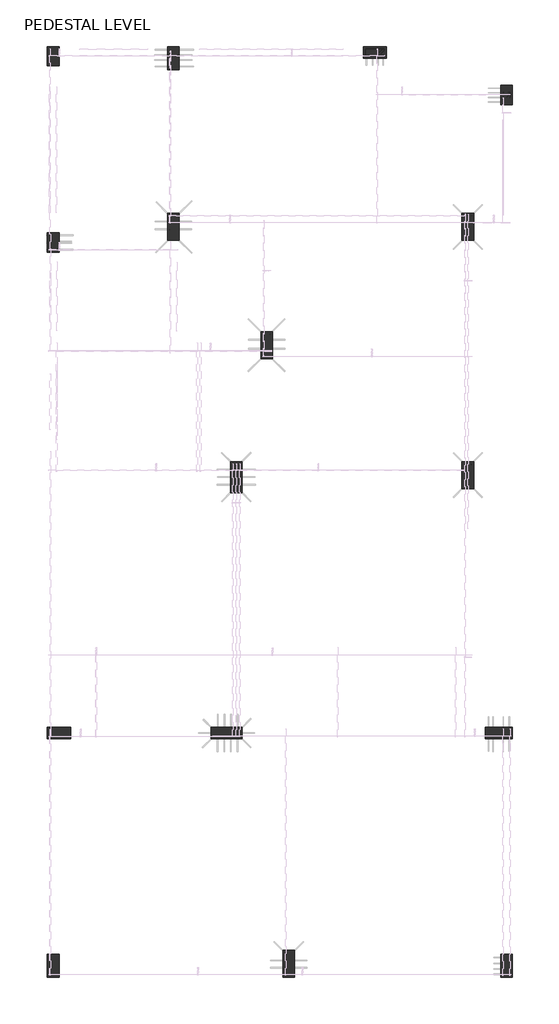
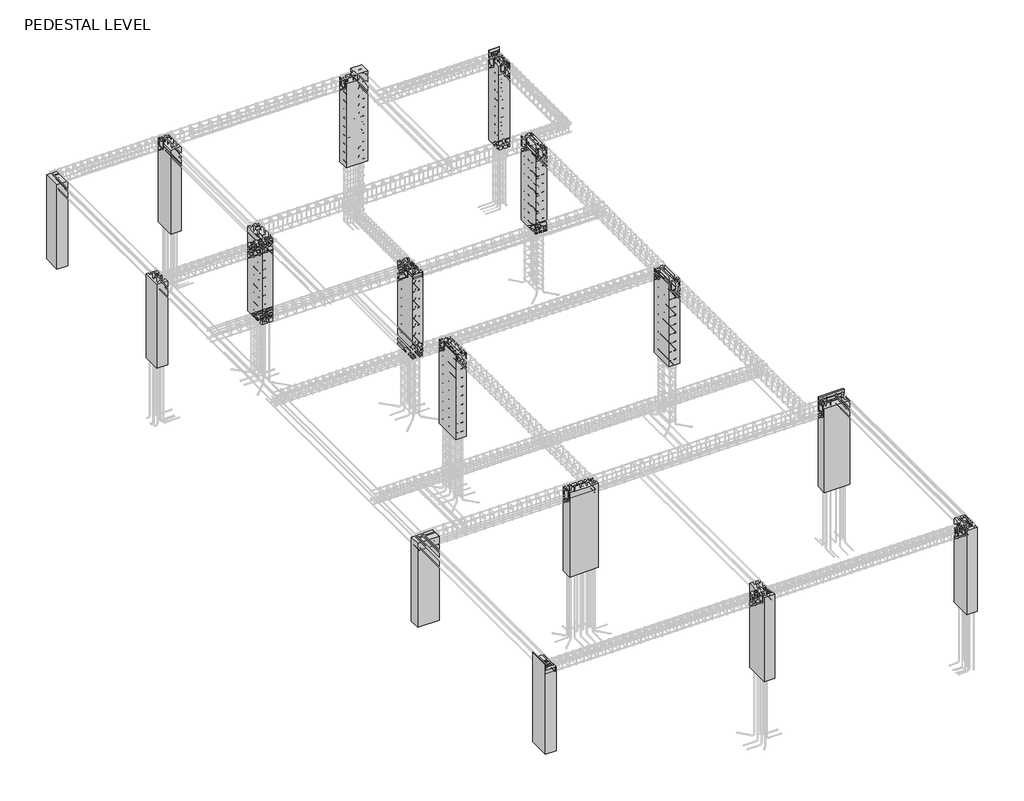
# One storey, part 1 of 8: 16 columns.
"""IFC4 building model written with IfcOpenShell, lengths in millimetres."""

from ifc_helpers import new_model, si_unit, origin, place, context, project, spatial, faceted_brep, element, save

model = new_model("IFC4")

# Units and contexts
model_context = context("Model", 3, world=origin())
ifc_project = project(units=[si_unit("LENGTHUNIT", "METRE", prefix="MILLI")], contexts=[model_context])

# Site, building, storey
site = spatial("IfcSite", under=ifc_project)
building = spatial("IfcBuilding", under=site)
storey = spatial("IfcBuildingStorey", under=building, Name="PEDESTAL LEVEL", Elevation=990.6)

# Columns
placement = place(None, origin())
element("IfcColumn", 1, ObjectType="Concrete-Rectangular-Column : C1", at=placement, inside=storey, context=model_context, shape_type="Brep", body=[
    faceted_brep([(150503.0232069, -91588.7007776, 990.6), (150503.0232069, -91969.7007776, 990.6), (150274.4232069, -91969.7007776, 990.6), (150274.4232069, -91588.7007776, 990.6), (150274.4232069, -91588.7007776, 2873.0), (150503.0232069, -91588.7007776, 2873.0), (150503.0232069, -91588.7007776, 2695.2), (150274.4232069, -91969.7007776, 2695.2), (150274.4232069, -91969.7007776, 2873.0), (150503.0232069, -91969.7007776, 2695.2), (150503.0232069, -91969.7007776, 2873.0), (150503.0232069, -91817.3007776, 2873.0)], [[[0, 1, 2, 3]], [[0, 3, 4, 5, 6]], [[3, 2, 7, 8, 4]], [[2, 1, 9, 10, 8, 7]], [[1, 0, 6, 5, 11, 10, 9]], [[5, 4, 8, 10, 11]]]),
])
element("IfcColumn", 2, ObjectType="Concrete-Rectangular-Column : C1", at=placement, inside=storey, context=model_context, shape_type="Brep", body=[
    faceted_brep([(159418.4232069, -92350.7007776, 3000.0), (159189.8232069, -92350.7007776, 3000.0), (159189.8232069, -92352.1871115, 3000.0), (159418.4232069, -92352.1871115, 3000.0), (159418.4232069, -92350.7007776, 990.6), (159418.4232069, -92731.7007776, 990.6), (159189.8232069, -92731.7007776, 990.6), (159189.8232069, -92350.7007776, 990.6), (159189.8232069, -92350.7007776, 2695.2), (159189.8232069, -92731.7007776, 2873.0), (159189.8232069, -92579.3007776, 2873.0), (159189.8232069, -92352.1871115, 2873.0), (159418.4232069, -92731.7007776, 2873.0), (159418.4232069, -92352.1871115, 2873.0)], [[[0, 1, 2, 3]], [[4, 5, 6, 7]], [[1, 0, 4, 7, 8]], [[7, 6, 9, 10, 11, 2, 1, 8]], [[6, 5, 12, 9]], [[5, 4, 0, 3, 13, 12]], [[13, 11, 10, 9, 12]], [[11, 13, 3, 2]]]),
])
element("IfcColumn", 3, ObjectType="Concrete-Rectangular-Column : C1", at=placement, inside=storey, context=model_context, shape_type="Brep", body=[
    faceted_brep([(150503.0232069, -95246.3007776, 990.6), (150503.0232069, -95627.3007776, 990.6), (150274.4232069, -95627.3007776, 990.6), (150274.4232069, -95246.3007776, 990.6), (150274.4232069, -95246.3007776, 2695.2), (150274.4232069, -95246.3007776, 2873.0), (150503.0232069, -95246.3007776, 2873.0), (150503.0232069, -95246.3007776, 2695.2), (150274.4232069, -95627.3007776, 2695.2), (150274.4232069, -95627.3007776, 2873.0), (150274.4232069, -95398.7007776, 2873.0), (150503.0232069, -95627.3007776, 2695.2), (150503.0232069, -95627.3007776, 2873.0), (150503.0232069, -95398.7007776, 2873.0)], [[[0, 1, 2, 3]], [[0, 3, 4, 5, 6, 7]], [[3, 2, 8, 9, 10, 5, 4]], [[2, 1, 11, 12, 9, 8]], [[1, 0, 7, 6, 13, 12, 11]], [[9, 12, 13, 6, 5, 10]]]),
])
element("IfcColumn", 4, ObjectType="Concrete-Rectangular-Column : C2", at=placement, inside=storey, context=model_context, shape_type="Brep", body=[
    faceted_brep([(152865.2232069, -91588.7007776, 990.6), (152865.2232069, -92045.9007776, 990.6), (152636.6232069, -92045.9007776, 990.6), (152636.6232069, -91588.7007776, 990.6), (152636.6232069, -91588.7007776, 2695.2), (152636.6232069, -91588.7007776, 2873.0), (152865.2232069, -91588.7007776, 2873.0), (152865.2232069, -91588.7007776, 2695.2), (152636.6232069, -92045.9007776, 2619.0), (152636.6232069, -92045.9007776, 2873.0), (152636.6232069, -91817.3007776, 2873.0), (152865.2232069, -92045.9007776, 2619.0), (152865.2232069, -92045.9007776, 2873.0), (152865.2232069, -91817.3007776, 2873.0)], [[[0, 1, 2, 3]], [[0, 3, 4, 5, 6, 7]], [[3, 2, 8, 9, 10, 5, 4]], [[2, 1, 11, 12, 9, 8]], [[1, 0, 7, 6, 13, 12, 11]], [[6, 5, 10, 9, 12, 13]]]),
])
element("IfcColumn", 5, ObjectType="Concrete-Rectangular-Column : C2", at=placement, inside=storey, context=model_context, shape_type="Brep", body=[
    faceted_brep([(156941.4384274, -91817.3007776, 3000.0), (156941.4384274, -91588.7007776, 3000.0), (156713.3232069, -91588.7007776, 3000.0), (156713.3232069, -91817.3007776, 3000.0), (156484.2384274, -91588.7007776, 990.6), (156941.4384274, -91588.7007776, 990.6), (156941.4384274, -91817.3007776, 990.6), (156484.2384274, -91817.3007776, 990.6), (156484.2384274, -91817.3007776, 2695.2), (156484.2384274, -91817.3007776, 2873.0), (156484.2384274, -91588.7007776, 2873.0), (156484.2384274, -91588.7007776, 2695.2), (156941.4384274, -91817.3007776, 2695.2), (156713.3232069, -91817.3007776, 2873.0), (156941.4384274, -91588.7007776, 2695.2), (156713.3232069, -91588.7007776, 2873.0)], [[[0, 1, 2, 3]], [[4, 5, 6, 7]], [[4, 7, 8, 9, 10, 11]], [[7, 6, 12, 0, 3, 13, 9, 8]], [[1, 0, 12, 6, 5, 14]], [[5, 4, 11, 10, 15, 2, 1, 14]], [[13, 15, 10, 9]], [[15, 13, 3, 2]]]),
])
element("IfcColumn", 6, ObjectType="Concrete-Rectangular-Column : C2", at=placement, inside=storey, context=model_context, shape_type="Brep", body=[
    faceted_brep([(150274.4232069, -104961.8007776, 990.6), (150731.6232069, -104961.8007776, 990.6), (150731.6232069, -105190.4007776, 990.6), (150274.4232069, -105190.4007776, 990.6), (150274.4232069, -105190.4007776, 2695.2), (150274.4232069, -105190.4007776, 2873.0), (150274.4232069, -104961.8007776, 2873.0), (150274.4232069, -104961.8007776, 2619.0), (150731.6232069, -105190.4007776, 2619.0), (150731.6232069, -105190.4007776, 2873.0), (150503.0232069, -105190.4007776, 2873.0), (150277.1537731, -105190.4007776, 2873.0), (150731.6232069, -104961.8007776, 2619.0), (150731.6232069, -104961.8007776, 2873.0), (150503.0232069, -104961.8007776, 2873.0)], [[[0, 1, 2, 3]], [[0, 3, 4, 5, 6, 7]], [[3, 2, 8, 9, 10, 11, 5, 4]], [[2, 1, 12, 13, 9, 8]], [[1, 0, 7, 6, 14, 13, 12]], [[6, 5, 11, 10, 9, 13, 14]]]),
])
element("IfcColumn", 7, ObjectType="Concrete-Rectangular-Column : C2", at=placement, inside=storey, context=model_context, shape_type="Brep", body=[
    faceted_brep([(159418.4232069, -109419.5007776, 990.6), (159418.4232069, -109876.7007776, 990.6), (159189.8232069, -109876.7007776, 990.6), (159189.8232069, -109419.5007776, 990.6), (159189.8232069, -109419.5007776, 2695.2), (159189.8232069, -109419.5007776, 2873.0), (159418.4232069, -109419.5007776, 2873.0), (159418.4232069, -109419.5007776, 2695.2), (159189.8232069, -109876.7007776, 2695.2), (159189.8232069, -109876.7007776, 2873.0), (159189.8232069, -109648.1007776, 2873.0), (159418.4232069, -109876.7007776, 2873.0)], [[[0, 1, 2, 3]], [[0, 3, 4, 5, 6, 7]], [[3, 2, 8, 9, 10, 5, 4]], [[2, 1, 11, 9, 8]], [[1, 0, 7, 6, 11]], [[6, 5, 10, 9, 11]]]),
])
element("IfcColumn", 8, ObjectType="Concrete-Rectangular-Column : C2", at=placement, inside=storey, context=model_context, shape_type="Brep", body=[
    faceted_brep([(150274.4232069, -109419.5007776, 3000.0), (150274.4232069, -109876.7007776, 3000.0), (150277.1537731, -109876.7007776, 3000.0), (150277.1537731, -109419.5007776, 3000.0), (150503.0232069, -109419.5007776, 990.6), (150503.0232069, -109876.7007776, 990.6), (150274.4232069, -109876.7007776, 990.6), (150274.4232069, -109419.5007776, 990.6), (150274.4232069, -109419.5007776, 2695.2), (150277.1537731, -109419.5007776, 2873.0), (150503.0232069, -109419.5007776, 2873.0), (150503.0232069, -109419.5007776, 2695.2), (150503.0232069, -109876.7007776, 2695.2), (150503.0232069, -109876.7007776, 2873.0), (150277.1537731, -109876.7007776, 2873.0), (150503.0232069, -109648.1007776, 2873.0)], [[[0, 1, 2, 3]], [[4, 5, 6, 7]], [[4, 7, 8, 0, 3, 9, 10, 11]], [[1, 0, 8, 7, 6]], [[6, 5, 12, 13, 14, 2, 1]], [[5, 4, 11, 10, 15, 13, 12]], [[9, 14, 13, 15, 10]], [[14, 9, 3, 2]]]),
])
element("IfcColumn", 9, ObjectType="Concrete-Rectangular-Column : C3", at=placement, inside=storey, context=model_context, shape_type="Brep", body=[
    faceted_brep([(158656.423207, -94865.3007776, 990.6), (158656.423207, -95398.7007776, 990.6), (158427.823207, -95398.7007776, 990.6), (158427.823207, -94865.3007776, 990.6), (158427.823207, -94865.3007776, 2619.0), (158427.823207, -94865.3007776, 2873.0), (158656.423207, -94865.3007776, 2873.0), (158656.423207, -94865.3007776, 2695.2), (158427.823207, -95398.7007776, 2619.0), (158427.823207, -95398.7007776, 2873.0), (158427.823207, -95093.9007776, 2873.0), (158656.423207, -95398.7007776, 2619.0), (158656.423207, -95398.7007776, 2873.0), (158656.423207, -95093.9007776, 2873.0)], [[[0, 1, 2, 3]], [[0, 3, 4, 5, 6, 7]], [[3, 2, 8, 9, 10, 5, 4]], [[2, 1, 11, 12, 9, 8]], [[1, 0, 7, 6, 13, 12, 11]], [[6, 5, 10, 9, 12, 13]]]),
])
element("IfcColumn", 10, ObjectType="Concrete-Rectangular-Column : C3", at=placement, inside=storey, context=model_context, shape_type="Brep", body=[
    faceted_brep([(158656.423207, -99742.1007776, 990.6), (158656.423207, -100275.5007776, 990.6), (158427.823207, -100275.5007776, 990.6), (158427.823207, -99742.1007776, 990.6), (158427.823207, -99742.1007776, 2619.0), (158427.823207, -99742.1007776, 2695.2), (158427.823207, -99742.1007776, 2873.0), (158656.423207, -99742.1007776, 2873.0), (158656.423207, -99742.1007776, 2619.0), (158427.823207, -100275.5007776, 2619.0), (158427.823207, -100275.5007776, 2873.0), (158427.823207, -99970.7007776, 2873.0), (158656.423207, -100275.5007776, 2619.0), (158656.423207, -100275.5007776, 2873.0), (158656.423207, -99970.7007776, 2873.0)], [[[0, 1, 2, 3]], [[0, 3, 4, 5, 6, 7, 8]], [[3, 2, 9, 10, 11, 6, 5, 4]], [[2, 1, 12, 13, 10, 9]], [[1, 0, 8, 7, 14, 13, 12]], [[7, 6, 11, 10, 13, 14]]]),
])
element("IfcColumn", 11, ObjectType="Concrete-Rectangular-Column : C3", at=placement, inside=storey, context=model_context, shape_type="Brep", body=[
    faceted_brep([(159418.4232069, -104961.8007776, 3000.0), (158885.0232069, -104961.8007776, 3000.0), (158885.0232069, -105001.8007776, 3000.0), (159418.4232069, -105001.8007776, 3000.0), (158885.0232069, -104961.8007776, 990.6), (159418.4232069, -104961.8007776, 990.6), (159418.4232069, -105190.4007776, 990.6), (158885.0232069, -105190.4007776, 990.6), (158885.0232069, -105190.4007776, 2619.0), (158885.0232069, -105190.4007776, 2873.0), (158885.0232069, -105001.8007776, 2873.0), (158885.0232069, -104961.8007776, 2619.0), (159418.4232069, -105190.4007776, 2873.0), (159418.4232069, -105001.8007776, 2873.0)], [[[0, 1, 2, 3]], [[4, 5, 6, 7]], [[4, 7, 8, 9, 10, 2, 1, 11]], [[7, 6, 12, 9, 8]], [[6, 5, 0, 3, 13, 12]], [[1, 0, 5, 4, 11]], [[13, 10, 9, 12]], [[10, 13, 3, 2]]]),
])
element("IfcColumn", 12, ObjectType="Concrete-Rectangular-Column : C4", at=placement, inside=storey, context=model_context, shape_type="Brep", body=[
    faceted_brep([(152865.2232069, -94865.3007776, 990.6), (152865.2232069, -95398.7007776, 990.6), (152636.6232069, -95398.7007776, 990.6), (152636.6232069, -94865.3007776, 990.6), (152636.6232069, -94865.3007776, 2619.0), (152636.6232069, -94865.3007776, 2873.0), (152865.2232069, -94865.3007776, 2873.0), (152865.2232069, -94865.3007776, 2619.0), (152636.6232069, -95398.7007776, 2695.2), (152636.6232069, -95398.7007776, 2873.0), (152636.6232069, -95093.9007776, 2873.0), (152865.2232069, -95398.7007776, 2695.2), (152865.2232069, -95398.7007776, 2873.0), (152865.2232069, -95093.9007776, 2873.0)], [[[0, 1, 2, 3]], [[0, 3, 4, 5, 6, 7]], [[3, 2, 8, 9, 10, 5, 4]], [[2, 1, 11, 12, 9, 8]], [[1, 0, 7, 6, 13, 12, 11]], [[6, 5, 10, 9, 12, 13]]]),
])
element("IfcColumn", 13, ObjectType="Concrete-Rectangular-Column : C4", at=placement, inside=storey, context=model_context, shape_type="Brep", body=[
    faceted_brep([(154699.7805846, -97189.4007776, 990.6), (154699.7805846, -97722.8007776, 990.6), (154471.1805846, -97722.8007776, 990.6), (154471.1805846, -97189.4007776, 990.6), (154471.1805846, -97189.4007776, 2695.2), (154471.1805846, -97189.4007776, 2873.0), (154699.7805846, -97189.4007776, 2873.0), (154699.7805846, -97189.4007776, 2695.2), (154471.1805846, -97722.8007776, 2873.0), (154699.7805846, -97722.8007776, 2695.2), (154699.7805846, -97722.8007776, 2873.0), (154699.7805846, -97494.2007776, 2873.0)], [[[0, 1, 2, 3]], [[0, 3, 4, 5, 6, 7]], [[3, 2, 8, 5, 4]], [[2, 1, 9, 10, 8]], [[1, 0, 7, 6, 11, 10, 9]], [[6, 5, 8, 10, 11]]]),
])
element("IfcColumn", 14, ObjectType="Concrete-Rectangular-Column : C4", at=placement, inside=storey, context=model_context, shape_type="Brep", body=[
    faceted_brep([(155132.1732069, -109343.3007776, 990.6), (155132.1732069, -109876.7007776, 990.6), (154903.5732069, -109876.7007776, 990.6), (154903.5732069, -109343.3007776, 990.6), (154903.5732069, -109343.3007776, 2695.2), (154903.5732069, -109343.3007776, 2873.0), (155132.1732069, -109343.3007776, 2873.0), (155132.1732069, -109343.3007776, 2695.2), (154903.5732069, -109876.7007776, 2695.2), (154903.5732069, -109876.7007776, 2873.0), (154903.5732069, -109648.1007776, 2873.0), (155132.1732069, -109876.7007776, 2695.2), (155132.1732069, -109876.7007776, 2873.0), (155132.1732069, -109648.1007776, 2873.0)], [[[0, 1, 2, 3]], [[0, 3, 4, 5, 6, 7]], [[3, 2, 8, 9, 10, 5, 4]], [[2, 1, 11, 12, 9, 8]], [[1, 0, 7, 6, 13, 12, 11]], [[6, 5, 10, 9, 12, 13]]]),
])
element("IfcColumn", 15, ObjectType="Concrete-Rectangular-Column : C5", at=placement, inside=storey, context=model_context, shape_type="Brep", body=[
    faceted_brep([(154102.8805846, -99742.1007776, 990.6), (154102.8805846, -100351.7007776, 990.6), (153874.2805846, -100351.7007776, 990.6), (153874.2805846, -99742.1007776, 990.6), (153874.2805846, -99742.1007776, 2873.0), (154102.8805846, -99742.1007776, 2873.0), (153874.2805846, -100351.7007776, 2695.2), (153874.2805846, -100351.7007776, 2873.0), (154102.8805846, -100351.7007776, 2695.2), (154102.8805846, -100351.7007776, 2873.0)], [[[0, 1, 2, 3]], [[0, 3, 4, 5]], [[3, 2, 6, 7, 4]], [[2, 1, 8, 9, 7, 6]], [[1, 0, 5, 9, 8]], [[5, 4, 7, 9]]]),
])
element("IfcColumn", 16, ObjectType="Concrete-Rectangular-Column : C6", at=placement, inside=storey, context=model_context, shape_type="Brep", body=[
    faceted_brep([(153493.2805846, -104961.8007776, 990.6), (154102.8805846, -104961.8007776, 990.6), (154102.8805846, -105190.4007776, 990.6), (153493.2805846, -105190.4007776, 990.6), (153493.2805846, -105190.4007776, 2619.0), (153493.2805846, -105190.4007776, 2873.0), (153493.2805846, -104961.8007776, 2873.0), (153493.2805846, -104961.8007776, 2619.0), (154102.8805846, -105190.4007776, 2619.0), (154102.8805846, -105190.4007776, 2873.0), (153867.9305846, -105190.4007776, 2873.0), (154102.8805846, -104961.8007776, 2619.0), (154102.8805846, -104961.8007776, 2695.2), (154102.8805846, -104961.8007776, 2873.0), (153874.2805846, -104961.8007776, 2873.0)], [[[0, 1, 2, 3]], [[0, 3, 4, 5, 6, 7]], [[3, 2, 8, 9, 10, 5, 4]], [[2, 1, 11, 12, 13, 9, 8]], [[1, 0, 7, 6, 14, 13, 12, 11]], [[9, 13, 14, 6, 5, 10]]]),
])

save(model, "model.ifc")

# Revit data of these elements
# Type "Concrete-Rectangular-Column : C1"
#   b = 228.6 mm
#   h = 381 mm
#   Structural Material [instance default] = Concrete, Cast-in-Place gray
# Type "Concrete-Rectangular-Column : C2"
#   b = 228.6 mm
#   h = 457.2 mm
#   Structural Material [instance default] = Concrete, Cast-in-Place gray
# Type "Concrete-Rectangular-Column : C3"
#   b = 228.6 mm
#   h = 533.4 mm
#   Structural Material [instance default] = Concrete, Cast-in-Place gray
# Type "Concrete-Rectangular-Column : C4"
#   b = 228.6 mm
#   h = 533.4 mm
#   Structural Material [instance default] = Concrete, Cast-in-Place gray
# Type "Concrete-Rectangular-Column : C5"
#   b = 228.6 mm
#   h = 609.6 mm
#   Structural Material [instance default] = Concrete, Cast-in-Place gray
# Type "Concrete-Rectangular-Column : C6"
#   b = 228.6 mm
#   h = 609.6 mm
#   Structural Material [instance default] = Concrete, Cast-in-Place gray
# Elements 1, 2, 3 (IfcColumn, "Concrete-Rectangular-Column : C1")
#   Structural Material = Concrete, Cast-in-Place gray
#   Phase Created = New Construction
#   Materials on its faces: "Concrete, Cast-in-Place gray"
# Elements 4, 5, 6, 7, 8 (IfcColumn, "Concrete-Rectangular-Column : C2")
#   Structural Material = Concrete, Cast-in-Place gray
#   Phase Created = New Construction
#   Materials on its faces: "Concrete, Cast-in-Place gray"
# Elements 9, 10, 11 (IfcColumn, "Concrete-Rectangular-Column : C3")
#   Structural Material = Concrete, Cast-in-Place gray
#   Phase Created = New Construction
#   Materials on its faces: "Concrete, Cast-in-Place gray"
# Elements 12, 13, 14 (IfcColumn, "Concrete-Rectangular-Column : C4")
#   Structural Material = Concrete, Cast-in-Place gray
#   Phase Created = New Construction
#   Materials on its faces: "Concrete, Cast-in-Place gray"
# Element 15 (IfcColumn, "Concrete-Rectangular-Column : C5")
#   Structural Material = Concrete, Cast-in-Place gray
#   Phase Created = New Construction
#   Materials on its faces: "Concrete, Cast-in-Place gray"
# Element 16 (IfcColumn, "Concrete-Rectangular-Column : C6")
#   Structural Material = Concrete, Cast-in-Place gray
#   Phase Created = New Construction
#   Materials on its faces: "Concrete, Cast-in-Place gray"
# Materials
#   "Concrete, Cast-in-Place gray": class "Concrete", colour RGB 192 192 192, transparency 0, Description = "Cast-in-place concrete", Cost = 0
